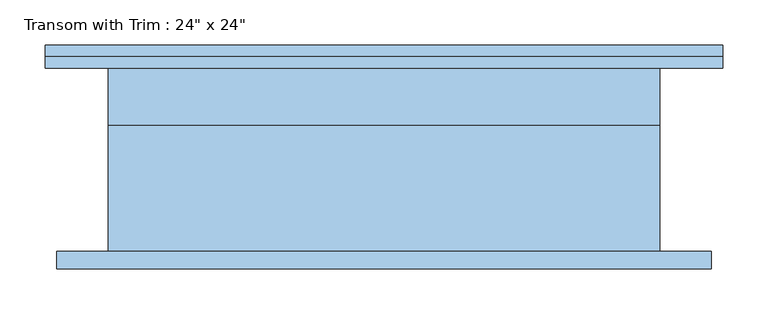
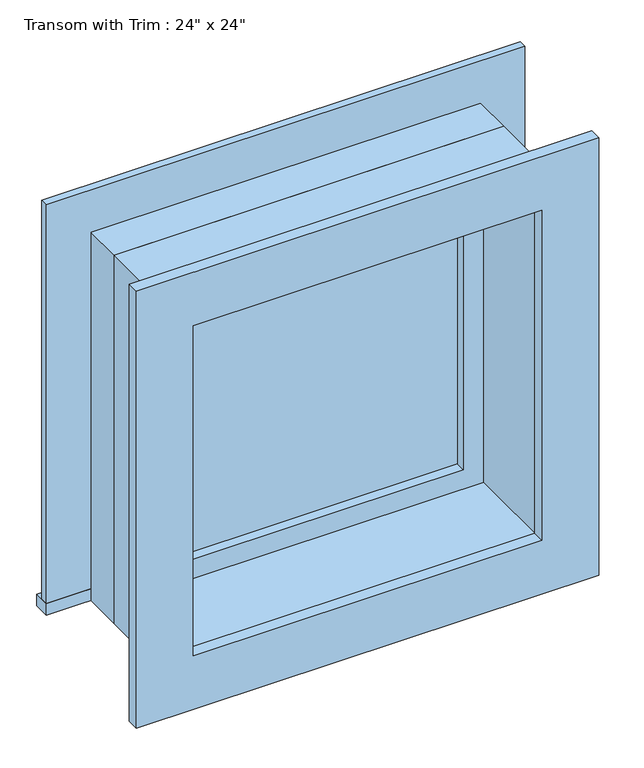
"""IFC4 building model written with IfcOpenShell, lengths in millimetres: window geometry."""

from ifc_helpers import new_model, si_unit, frame, origin, place, context, project, spatial, polyline, outline, extrude, source, transform, mapped, element, save


def window_e41d21a6(model_context):
    return source(origin(), model_context, "Body", "SweptSolid", [
        extrude(outline(polyline([(-412.75, 127.0), (336.55, 127.0), (336.55, 101.6), (-412.75, 101.6), (-412.75, 127.0)])), frame((0.0, 0.0, 2159.0), z_axis=(0.0, 0.0, 1.0), x_axis=(1.0, 0.0, 0.0)), (0.0, 0.0, 1.0), 19.05),
        extrude(outline(polyline([(2749.55, -323.85), (2749.55, 247.65), (2178.05, 247.65), (2178.05, 336.55), (2838.45, 336.55), (2838.45, -412.75), (2178.05, -412.75), (2178.05, -323.85), (2749.55, -323.85)])), frame((0.0, 101.6, 0.0), z_axis=(0.0, 1.0, 0.0), x_axis=(0.0, 0.0, 1.0)), (0.0, 0.0, 1.0), 12.7),
        extrude(outline(polyline([(2825.75, 323.85), (2825.75, -400.05), (2101.85, -400.05), (2101.85, 323.85), (2825.75, 323.85)]), holes=[polyline([(2736.85, 234.95), (2190.75, 234.95), (2190.75, -311.15), (2736.85, -311.15), (2736.85, 234.95)])]), frame((0.0, -120.65, 0.0), z_axis=(0.0, 1.0, 0.0), x_axis=(0.0, 0.0, 1.0)), (0.0, 0.0, 1.0), 19.05),
        extrude(outline(polyline([(203.2, 53.975), (-279.4, 53.975), (-279.4, 66.675), (203.2, 66.675), (203.2, 53.975)])), frame((0.0, 0.0, 2222.5), z_axis=(0.0, 0.0, 1.0), x_axis=(1.0, 0.0, 0.0)), (0.0, 0.0, 1.0), 482.6),
        extrude(outline(polyline([(2749.55, -323.85), (2178.05, -323.85), (2178.05, 247.65), (2749.55, 247.65), (2749.55, -323.85)]), holes=[polyline([(2705.1, -279.4), (2705.1, 203.2), (2222.5, 203.2), (2222.5, -279.4), (2705.1, -279.4)])]), frame((0.0, 38.1, 0.0), z_axis=(0.0, 1.0, 0.0), x_axis=(0.0, 0.0, 1.0)), (0.0, 0.0, 1.0), 44.45),
        extrude(outline(polyline([(2768.6, -342.9), (2159.0, -342.9), (2159.0, 266.7), (2768.6, 266.7), (2768.6, -342.9)]), holes=[polyline([(2736.85, -311.15), (2736.85, 234.95), (2190.75, 234.95), (2190.75, -311.15), (2736.85, -311.15)])]), frame((0.0, -101.6, 0.0), z_axis=(0.0, 1.0, 0.0), x_axis=(0.0, 0.0, 1.0)), (0.0, 0.0, 1.0), 139.7),
        extrude(outline(polyline([(2768.6, 266.7), (2768.6, -342.9), (2159.0, -342.9), (2159.0, 266.7), (2768.6, 266.7)]), holes=[polyline([(2749.55, 247.65), (2178.05, 247.65), (2178.05, -323.85), (2749.55, -323.85), (2749.55, 247.65)])]), frame((0.0, 38.1, 0.0), z_axis=(0.0, 1.0, 0.0), x_axis=(0.0, 0.0, 1.0)), (0.0, 0.0, 1.0), 63.5),
    ])


if __name__ == "__main__":
    model = new_model("IFC4")
    model_context = context("Model", 3, world=origin())
    ifc_project = project(units=[si_unit("LENGTHUNIT", "METRE", prefix="MILLI")], contexts=[model_context])
    site = spatial("IfcSite", under=ifc_project)
    building = spatial("IfcBuilding", under=site)
    placement = place(None, origin())
    window_shape = window_e41d21a6(model_context)
    element("IfcWindow", 1, ObjectType="Transom with Trim : 24\" x 24\"", at=placement, inside=building, context=model_context, shape_type="MappedRepresentation", body=[
        mapped(window_shape, transform((0.0, 0.0, 0.0), x_axis=(1.0, 0.0, 0.0), y_axis=(0.0, 1.0, 0.0), z_axis=(0.0, 0.0, 1.0))),
    ])
    save(model, "model.ifc")

# Revit data of these elements
# Type "Transom with Trim : 24\" x 24\""
#   Type Mark = "16"
#   Construction Type Id = "GSP4R"
#   Assembly Code = "B2020100"
#   Analytic Construction = "1/8 in Pilkington single glazing"
#   Visual Light Transmittance = 0.9
#   Solar Heat Gain Coefficient = 0.78
#   Heat Transfer Coefficient (U) = 0.6496 BTU/(h·ft²·°F)
#   Height = 2' - 0"
#   Default Sill Height = 7' - 1"
#   Trim Projection - Ext. = 0' - 0 1/2"
#   Trim Projection - Int. = 0' - 0 3/4"
#   Trim Width - Exterior = 0' - 3 1/2"
#   Trim Width - Interior = 0' - 3 1/2"
#   Width = 2' - 0"
#   Window Inset = 0' - 0 3/4"
#   Define Thermal Properties by = 1
#   Glass Pane Material = Glass
#   Sash Material = Sash
#   Trim Exterior Material = Trim
#   Trim Interior Material = Trim
#   Wall Closure = (empty or 0)
# Element 1 (IfcWindow, "Transom with Trim : 24\" x 24\"")
#   Materials on its faces: "Sash", "Trim", "Glass"
# Materials
#   "Glass": class "Glass", colour RGB 0 128 192, transparency 0.75, Description = "Soda Lime Glass", Cost = 0
#   "Sash": class "Wood", colour RGB 224 178 126, transparency 0
#   "Trim": class "Wood", colour RGB 224 178 126, transparency 0
